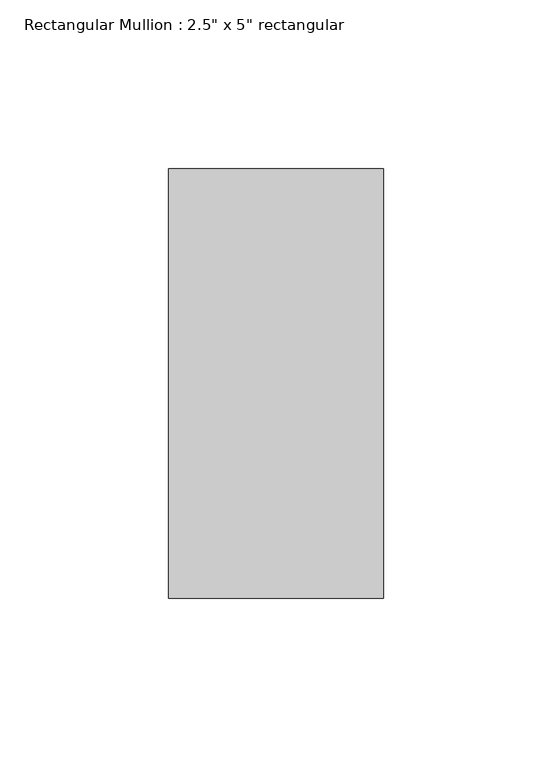
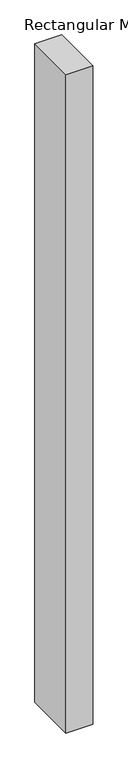
"""IFC4 building model written with IfcOpenShell, lengths in millimetres: member geometry."""

from ifc_helpers import new_model, si_unit, frame, origin, place, context, project, spatial, polyline, outline, extrude, source, transform, mapped, element, save


def member_24084ae4(model_context):
    return source(origin(), model_context, "Body", "SweptSolid", [
        extrude(outline(polyline([(0.0, 63.5), (0.0, -63.5), (-63.5, -63.5), (-63.5, 63.5), (0.0, 63.5)])), frame((0.0, 0.0, -1644.7338557), z_axis=(0.0, 0.0, 1.0), x_axis=(1.0, 0.0, 0.0)), (0.0, 0.0, 1.0), 1644.7338557),
    ])


if __name__ == "__main__":
    model = new_model("IFC4")
    model_context = context("Model", 3, world=origin())
    ifc_project = project(units=[si_unit("LENGTHUNIT", "METRE", prefix="MILLI")], contexts=[model_context])
    site = spatial("IfcSite", under=ifc_project)
    building = spatial("IfcBuilding", under=site)
    placement = place(None, origin())
    member_shape = member_24084ae4(model_context)
    element("IfcMember", 1, ObjectType="Rectangular Mullion : 2.5\" x 5\" rectangular", at=placement, inside=building, context=model_context, shape_type="MappedRepresentation", body=[
        mapped(member_shape, transform((0.0, 0.0, 0.0), x_axis=(1.0, 0.0, 0.0), y_axis=(0.0, 1.0, 0.0), z_axis=(0.0, 0.0, 1.0))),
    ])
    save(model, "model.ifc")

# Revit data of these elements
# Type "Rectangular Mullion : 2.5\" x 5\" rectangular"
#   built-in parameter 1007304 = 0.416667 (stored number, unit not read)
#   built-in parameter 1007301 = 0.104167 (stored number, unit not read)
#   built-in parameter 1007300 = 0.104167 (stored number, unit not read)
# Element 1 (IfcMember, "Rectangular Mullion : 2.5\" x 5\" rectangular")
#   Materials on its faces: "Aluminum"
# Materials
#   "Aluminum": class "Metal", colour RGB 247 247 247, transparency 0, Description = "Aluminum 6061", Cost = 0
